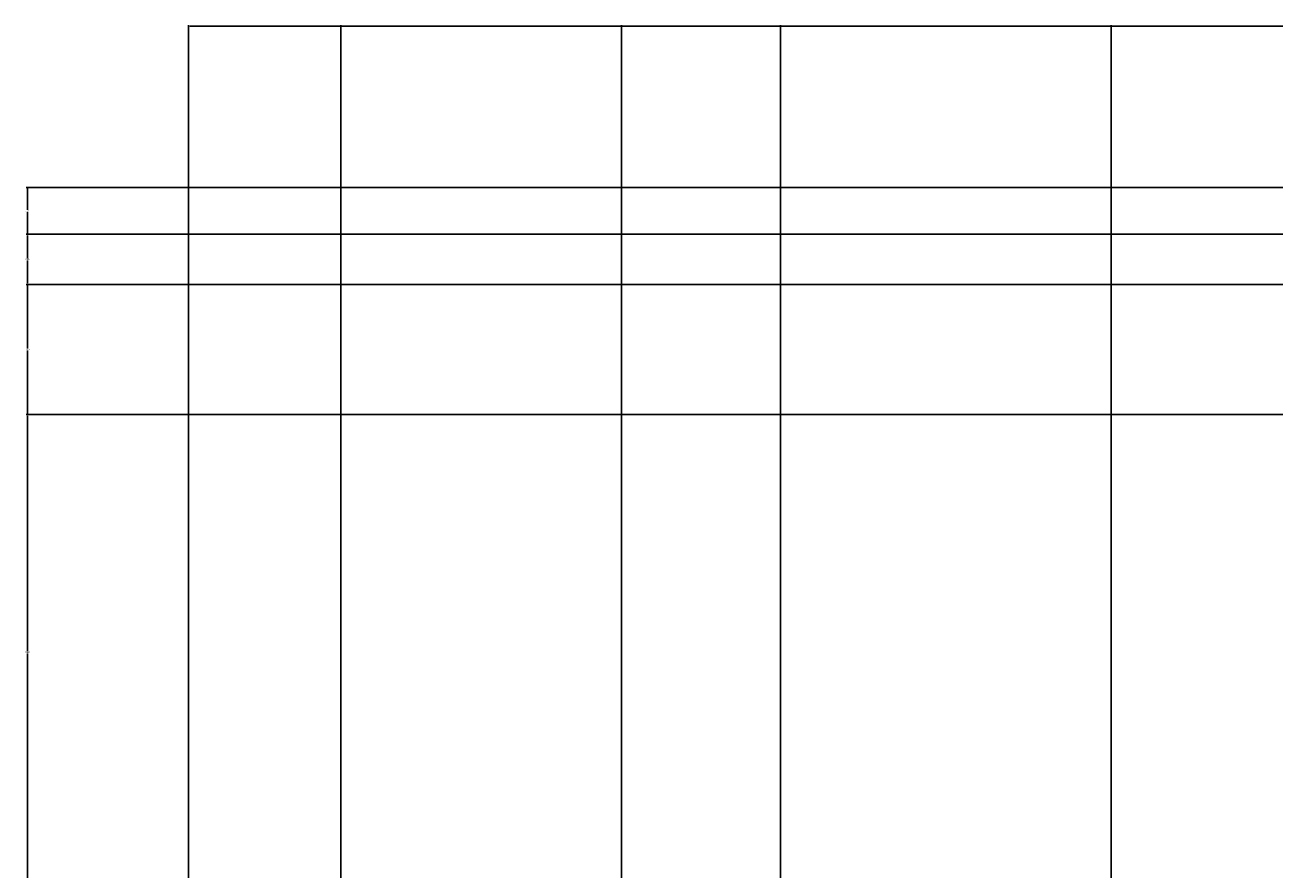
# Model space of a CAD drawing. Units: inches. Extents: x 93 to 565, y 123 to 656.
# Tile 8 of 18: x 93 to 291, y 522 to 656. Entities that reach past the tile are written whole.
import ezdxf

# ---------------------------------------------------------------- set-up
doc = ezdxf.new("R2010")
doc.units = ezdxf.units.IN
doc.header["$MEASUREMENT"] = 0
doc.layers.add('A-ANNO-DIMS', color=2, linetype='Continuous', lineweight=18)
doc.styles.get("Standard").update_dxf_attribs({"font": 'arial.ttf'})
doc.dimstyles.get("Standard").update_dxf_attribs({"dimtxt": 0.18, "dimasz": 0.18, "dimexe": 0.18, "dimexo": 0.0625, "dimgap": 0.09, "dimtad": 0, "dimtih": 1, "dimtoh": 1, "dimdec": 4, "dimzin": 0, "dimdsep": 46, "dimtxsty": 'Standard', "dimcen": 0.09, "dimadec": 0, "dimazin": 0, "dimtfac": 1, "dimtdec": 4, "dimtofl": 0, "dimtmove": 0, "dimatfit": 3, "dimfxl": 1, "dimtolj": 1, "dimtzin": 0, "dimarcsym": 0})

# ---------------------------------------------------------------- blocks, each defined once
blk = doc.blocks.new('*D26')
at = {"layer": 'A-ANNO-DIMS', "color": 0, "lineweight": -2, "transparency": 16777216}
for p, q in [((119.08, 519.16), (119.08, 656.13)), ((119.26, 655.95), (328.79, 655.95)), ((538.9, 655.95), (329.37, 655.95)), ((539.08, 630.47), (539.08, 656.13))]:
    blk.add_line(p, q, dxfattribs=at)
at = {"layer": 'A-ANNO-DIMS', "color": 0, "transparency": 16777216}
for points in [[(119.26, 655.98), (119.26, 655.92), (119.08, 655.95)], [(538.9, 655.98), (538.9, 655.92), (539.08, 655.95)]]:
    blk.add_solid(points, dxfattribs=at)
at = {"layer": 'Defpoints', "color": 0, "transparency": 16777216}
for p in [(539.08, 655.95), (539.08, 630.4), (119.08, 519.1)]:
    blk.add_point(p, dxfattribs=at)
at = {"layer": 'A-ANNO-DIMS', "color": 0, "transparency": 16777216, "insert": (329.08, 655.95), "char_height": 0.18, "attachment_point": 5}
blk.add_mtext('\\A1;420', dxfattribs=at)
blk = doc.blocks.new('*D31')
at = {"layer": 'A-ANNO-DIMS', "color": 0, "lineweight": -2, "transparency": 16777216}
for p, q in [((417.87, 630.4), (564.81, 630.4)), ((564.63, 630.22), (564.63, 395.25)), ((564.63, 159.91), (564.63, 394.89)), ((119.14, 159.73), (564.81, 159.73))]:
    blk.add_line(p, q, dxfattribs=at)
at = {"layer": 'A-ANNO-DIMS', "color": 0, "transparency": 16777216}
for points in [[(564.6, 630.22), (564.66, 630.22), (564.63, 630.4)], [(564.6, 159.91), (564.66, 159.91), (564.63, 159.73)]]:
    blk.add_solid(points, dxfattribs=at)
at = {"layer": 'Defpoints', "color": 0, "transparency": 16777216}
for p in [(417.81, 630.4), (564.63, 630.4), (119.08, 159.73)]:
    blk.add_point(p, dxfattribs=at)
at = {"layer": 'A-ANNO-DIMS', "color": 0, "transparency": 16777216, "insert": (564.63, 395.07), "char_height": 0.18, "attachment_point": 5}
blk.add_mtext('\\A1;470.7', dxfattribs=at)
blk = doc.blocks.new('*D36')
at = {"layer": 'A-ANNO-DIMS', "color": 0, "lineweight": -2, "transparency": 16777216}
for p, q in [((417.75, 594.4), (93.35, 594.4)), ((93.53, 594.22), (93.53, 556.93)), ((93.53, 519.28), (93.53, 556.57)), ((119.02, 519.1), (93.35, 519.1))]:
    blk.add_line(p, q, dxfattribs=at)
at = {"layer": 'A-ANNO-DIMS', "color": 0, "transparency": 16777216}
for points in [[(93.5, 594.22), (93.56, 594.22), (93.53, 594.4)], [(93.5, 519.28), (93.56, 519.28), (93.53, 519.1)]]:
    blk.add_solid(points, dxfattribs=at)
at = {"layer": 'Defpoints', "color": 0, "transparency": 16777216}
for p in [(93.53, 594.4), (417.81, 594.4), (119.08, 519.1)]:
    blk.add_point(p, dxfattribs=at)
at = {"layer": 'A-ANNO-DIMS', "color": 0, "transparency": 16777216, "insert": (93.53, 556.75), "char_height": 0.18, "attachment_point": 5}
blk.add_mtext('\\A1;75.3', dxfattribs=at)
blk = doc.blocks.new('*D49')
at = {"layer": 'A-ANNO-DIMS', "color": 0, "lineweight": -2, "transparency": 16777216}
for p, q in [((119.08, 519.16), (119.08, 656.13)), ((119.26, 655.95), (130.75, 655.95)), ((143.03, 655.95), (131.54, 655.95)), ((143.21, 494.41), (143.21, 656.13))]:
    blk.add_line(p, q, dxfattribs=at)
at = {"layer": 'A-ANNO-DIMS', "color": 0, "transparency": 16777216}
for points in [[(119.26, 655.98), (119.26, 655.92), (119.08, 655.95)], [(143.03, 655.98), (143.03, 655.92), (143.21, 655.95)]]:
    blk.add_solid(points, dxfattribs=at)
at = {"layer": 'Defpoints', "color": 0, "transparency": 16777216}
for p in [(143.21, 655.95), (119.08, 519.1), (143.21, 494.34)]:
    blk.add_point(p, dxfattribs=at)
at = {"layer": 'A-ANNO-DIMS', "color": 0, "transparency": 16777216, "insert": (131.15, 655.95), "char_height": 0.18, "attachment_point": 5}
blk.add_mtext('\\A1;24.13', dxfattribs=at)
blk = doc.blocks.new('*D50')
at = {"layer": 'A-ANNO-DIMS', "color": 0, "lineweight": -2, "transparency": 16777216}
for p, q in [((143.21, 494.41), (143.21, 656.13)), ((143.39, 655.95), (165.03, 655.95)), ((187.47, 655.95), (165.83, 655.95)), ((187.65, 494.41), (187.65, 656.13))]:
    blk.add_line(p, q, dxfattribs=at)
at = {"layer": 'A-ANNO-DIMS', "color": 0, "transparency": 16777216}
for points in [[(143.39, 655.98), (143.39, 655.92), (143.21, 655.95)], [(187.47, 655.98), (187.47, 655.92), (187.65, 655.95)]]:
    blk.add_solid(points, dxfattribs=at)
at = {"layer": 'Defpoints', "color": 0, "transparency": 16777216}
for p in [(187.65, 655.95), (143.21, 494.34), (187.65, 494.34)]:
    blk.add_point(p, dxfattribs=at)
at = {"layer": 'A-ANNO-DIMS', "color": 0, "transparency": 16777216, "insert": (165.43, 655.95), "char_height": 0.18, "attachment_point": 5}
blk.add_mtext('\\A1;44.44', dxfattribs=at)
blk = doc.blocks.new('*D64')
at = {"layer": 'A-ANNO-DIMS', "color": 0, "lineweight": -2, "transparency": 16777216}
for p, q in [((212.83, 427.41), (212.83, 656.13)), ((213.01, 655.95), (238.63, 655.95)), ((265.03, 655.95), (239.41, 655.95)), ((265.21, 427.41), (265.21, 656.13))]:
    blk.add_line(p, q, dxfattribs=at)
at = {"layer": 'A-ANNO-DIMS', "color": 0, "transparency": 16777216}
for points in [[(213.01, 655.98), (213.01, 655.92), (212.83, 655.95)], [(265.03, 655.98), (265.03, 655.92), (265.21, 655.95)]]:
    blk.add_solid(points, dxfattribs=at)
at = {"layer": 'Defpoints', "color": 0, "transparency": 16777216}
for p in [(265.21, 655.95), (212.83, 427.35), (265.21, 427.35)]:
    blk.add_point(p, dxfattribs=at)
at = {"layer": 'A-ANNO-DIMS', "color": 0, "transparency": 16777216, "insert": (239.02, 655.95), "char_height": 0.18, "attachment_point": 5}
blk.add_mtext('\\A1;52.39', dxfattribs=at)
blk = doc.blocks.new('*D94')
at = {"layer": 'A-ANNO-DIMS', "color": 0, "lineweight": -2, "transparency": 16777216}
for p, q in [((423.75, 615.04), (93.35, 615.04)), ((93.53, 614.86), (93.53, 604.9)), ((93.53, 594.58), (93.53, 604.54)), ((417.75, 594.4), (93.35, 594.4))]:
    blk.add_line(p, q, dxfattribs=at)
at = {"layer": 'A-ANNO-DIMS', "color": 0, "transparency": 16777216}
for points in [[(93.5, 614.86), (93.56, 614.86), (93.53, 615.04)], [(93.5, 594.58), (93.56, 594.58), (93.53, 594.4)]]:
    blk.add_solid(points, dxfattribs=at)
at = {"layer": 'Defpoints', "color": 0, "transparency": 16777216}
for p in [(93.53, 615.04), (423.81, 615.04), (417.81, 594.4)]:
    blk.add_point(p, dxfattribs=at)
at = {"layer": 'A-ANNO-DIMS', "color": 0, "transparency": 16777216, "insert": (93.53, 604.72), "char_height": 0.18, "attachment_point": 5}
blk.add_mtext('\\A1;20.636', dxfattribs=at)
blk = doc.blocks.new('*D95')
at = {"layer": 'A-ANNO-DIMS', "color": 0, "lineweight": -2, "transparency": 16777216}
for p, q in [((487.73, 622.97), (93.35, 622.97)), ((93.53, 622.79), (93.53, 619.19)), ((93.53, 615.22), (93.53, 618.82)), ((423.75, 615.04), (93.35, 615.04))]:
    blk.add_line(p, q, dxfattribs=at)
at = {"layer": 'A-ANNO-DIMS', "color": 0, "transparency": 16777216}
for points in [[(93.5, 622.79), (93.56, 622.79), (93.53, 622.97)], [(93.5, 615.22), (93.56, 615.22), (93.53, 615.04)]]:
    blk.add_solid(points, dxfattribs=at)
at = {"layer": 'Defpoints', "color": 0, "transparency": 16777216}
for p in [(93.53, 622.97), (487.8, 622.97), (423.81, 615.04)]:
    blk.add_point(p, dxfattribs=at)
at = {"layer": 'A-ANNO-DIMS', "color": 0, "transparency": 16777216, "insert": (93.53, 619.01), "char_height": 0.18, "attachment_point": 5}
blk.add_mtext('\\A1;7.93', dxfattribs=at)
blk = doc.blocks.new('*D96')
at = {"layer": 'A-ANNO-DIMS', "color": 0, "lineweight": -2, "transparency": 16777216}
for p, q in [((417.75, 630.4), (93.35, 630.4)), ((93.53, 630.22), (93.53, 626.87)), ((93.53, 623.15), (93.53, 626.51)), ((487.73, 622.97), (93.35, 622.97))]:
    blk.add_line(p, q, dxfattribs=at)
at = {"layer": 'A-ANNO-DIMS', "color": 0, "transparency": 16777216}
for points in [[(93.5, 630.22), (93.56, 630.22), (93.53, 630.4)], [(93.5, 623.15), (93.56, 623.15), (93.53, 622.97)]]:
    blk.add_solid(points, dxfattribs=at)
at = {"layer": 'Defpoints', "color": 0, "transparency": 16777216}
for p in [(93.53, 630.4), (417.81, 630.4), (487.8, 622.97)]:
    blk.add_point(p, dxfattribs=at)
at = {"layer": 'A-ANNO-DIMS', "color": 0, "transparency": 16777216, "insert": (93.53, 626.69), "char_height": 0.18, "attachment_point": 5}
blk.add_mtext('\\A1;7.434', dxfattribs=at)
blk = doc.blocks.new('*D105')
at = {"layer": 'A-ANNO-DIMS', "color": 0, "lineweight": -2, "transparency": 16777216}
for p, q in [((119.08, 519.16), (119.08, 656.13)), ((119.26, 655.95), (328.54, 655.95)), ((538.9, 655.95), (329.62, 655.95)), ((539.08, 630.47), (539.08, 656.13))]:
    blk.add_line(p, q, dxfattribs=at)
at = {"layer": 'A-ANNO-DIMS', "color": 0, "transparency": 16777216}
for points in [[(119.26, 655.98), (119.26, 655.92), (119.08, 655.95)], [(538.9, 655.98), (538.9, 655.92), (539.08, 655.95)]]:
    blk.add_solid(points, dxfattribs=at)
at = {"layer": 'Defpoints', "color": 0, "transparency": 16777216}
for p in [(539.08, 655.95), (539.08, 630.4), (119.08, 519.1)]:
    blk.add_point(p, dxfattribs=at)
at = {"layer": 'A-ANNO-DIMS', "color": 0, "transparency": 16777216, "insert": (329.08, 655.95), "char_height": 0.18, "attachment_point": 5}
blk.add_mtext('\\A1;420.000', dxfattribs=at)
blk = doc.blocks.new('*D110')
at = {"layer": 'A-ANNO-DIMS', "color": 0, "lineweight": -2, "transparency": 16777216}
for p, q in [((417.87, 630.4), (564.81, 630.4)), ((564.63, 630.22), (564.63, 395.25)), ((564.63, 159.91), (564.63, 394.89)), ((119.14, 159.73), (564.81, 159.73))]:
    blk.add_line(p, q, dxfattribs=at)
at = {"layer": 'A-ANNO-DIMS', "color": 0, "transparency": 16777216}
for points in [[(564.6, 630.22), (564.66, 630.22), (564.63, 630.4)], [(564.6, 159.91), (564.66, 159.91), (564.63, 159.73)]]:
    blk.add_solid(points, dxfattribs=at)
at = {"layer": 'Defpoints', "color": 0, "transparency": 16777216}
for p in [(417.81, 630.4), (564.63, 630.4), (119.08, 159.73)]:
    blk.add_point(p, dxfattribs=at)
at = {"layer": 'A-ANNO-DIMS', "color": 0, "transparency": 16777216, "insert": (564.63, 395.07), "char_height": 0.18, "attachment_point": 5}
blk.add_mtext('\\A1;470.673', dxfattribs=at)
blk = doc.blocks.new('*D115')
at = {"layer": 'A-ANNO-DIMS', "color": 0, "lineweight": -2, "transparency": 16777216}
for p, q in [((417.75, 594.4), (93.35, 594.4)), ((93.53, 594.22), (93.53, 556.93)), ((93.53, 519.28), (93.53, 556.57)), ((119.02, 519.1), (93.35, 519.1))]:
    blk.add_line(p, q, dxfattribs=at)
at = {"layer": 'A-ANNO-DIMS', "color": 0, "transparency": 16777216}
for points in [[(93.5, 594.22), (93.56, 594.22), (93.53, 594.4)], [(93.5, 519.28), (93.56, 519.28), (93.53, 519.1)]]:
    blk.add_solid(points, dxfattribs=at)
at = {"layer": 'Defpoints', "color": 0, "transparency": 16777216}
for p in [(93.53, 594.4), (417.81, 594.4), (119.08, 519.1)]:
    blk.add_point(p, dxfattribs=at)
at = {"layer": 'A-ANNO-DIMS', "color": 0, "transparency": 16777216, "insert": (93.53, 556.75), "char_height": 0.18, "attachment_point": 5}
blk.add_mtext('\\A1;75.305', dxfattribs=at)
blk = doc.blocks.new('*D128')
at = {"layer": 'A-ANNO-DIMS', "color": 0, "lineweight": -2, "transparency": 16777216}
for p, q in [((119.08, 519.16), (119.08, 656.13)), ((119.26, 655.95), (130.68, 655.95)), ((143.03, 655.95), (131.61, 655.95)), ((143.21, 494.41), (143.21, 656.13))]:
    blk.add_line(p, q, dxfattribs=at)
at = {"layer": 'A-ANNO-DIMS', "color": 0, "transparency": 16777216}
for points in [[(119.26, 655.98), (119.26, 655.92), (119.08, 655.95)], [(143.03, 655.98), (143.03, 655.92), (143.21, 655.95)]]:
    blk.add_solid(points, dxfattribs=at)
at = {"layer": 'Defpoints', "color": 0, "transparency": 16777216}
for p in [(143.21, 655.95), (119.08, 519.1), (143.21, 494.34)]:
    blk.add_point(p, dxfattribs=at)
at = {"layer": 'A-ANNO-DIMS', "color": 0, "transparency": 16777216, "insert": (131.15, 655.95), "char_height": 0.18, "attachment_point": 5}
blk.add_mtext('\\A1;24.132', dxfattribs=at)
blk = doc.blocks.new('*D129')
at = {"layer": 'A-ANNO-DIMS', "color": 0, "lineweight": -2, "transparency": 16777216}
for p, q in [((143.21, 494.41), (143.21, 656.13)), ((143.39, 655.95), (164.96, 655.95)), ((187.47, 655.95), (165.9, 655.95)), ((187.65, 494.41), (187.65, 656.13))]:
    blk.add_line(p, q, dxfattribs=at)
at = {"layer": 'A-ANNO-DIMS', "color": 0, "transparency": 16777216}
for points in [[(143.39, 655.98), (143.39, 655.92), (143.21, 655.95)], [(187.47, 655.98), (187.47, 655.92), (187.65, 655.95)]]:
    blk.add_solid(points, dxfattribs=at)
at = {"layer": 'Defpoints', "color": 0, "transparency": 16777216}
for p in [(187.65, 655.95), (143.21, 494.34), (187.65, 494.34)]:
    blk.add_point(p, dxfattribs=at)
at = {"layer": 'A-ANNO-DIMS', "color": 0, "transparency": 16777216, "insert": (165.43, 655.95), "char_height": 0.18, "attachment_point": 5}
blk.add_mtext('\\A1;44.436', dxfattribs=at)
blk = doc.blocks.new('*D143')
at = {"layer": 'A-ANNO-DIMS', "color": 0, "lineweight": -2, "transparency": 16777216}
for p, q in [((212.83, 427.41), (212.83, 656.13)), ((213.01, 655.95), (238.56, 655.95)), ((265.03, 655.95), (239.48, 655.95)), ((265.21, 427.41), (265.21, 656.13))]:
    blk.add_line(p, q, dxfattribs=at)
at = {"layer": 'A-ANNO-DIMS', "color": 0, "transparency": 16777216}
for points in [[(213.01, 655.98), (213.01, 655.92), (212.83, 655.95)], [(265.03, 655.98), (265.03, 655.92), (265.21, 655.95)]]:
    blk.add_solid(points, dxfattribs=at)
at = {"layer": 'Defpoints', "color": 0, "transparency": 16777216}
for p in [(265.21, 655.95), (212.83, 427.35), (265.21, 427.35)]:
    blk.add_point(p, dxfattribs=at)
at = {"layer": 'A-ANNO-DIMS', "color": 0, "transparency": 16777216, "insert": (239.02, 655.95), "char_height": 0.18, "attachment_point": 5}
blk.add_mtext('\\A1;52.388', dxfattribs=at)
blk = doc.blocks.new('*D173')
at = {"layer": 'A-ANNO-DIMS', "color": 0, "lineweight": -2, "transparency": 16777216}
for p, q in [((423.75, 615.04), (93.35, 615.04)), ((93.53, 614.86), (93.53, 604.9)), ((93.53, 594.58), (93.53, 604.54)), ((417.75, 594.4), (93.35, 594.4))]:
    blk.add_line(p, q, dxfattribs=at)
at = {"layer": 'A-ANNO-DIMS', "color": 0, "transparency": 16777216}
for points in [[(93.5, 614.86), (93.56, 614.86), (93.53, 615.04)], [(93.5, 594.58), (93.56, 594.58), (93.53, 594.4)]]:
    blk.add_solid(points, dxfattribs=at)
at = {"layer": 'Defpoints', "color": 0, "transparency": 16777216}
for p in [(93.53, 615.04), (423.81, 615.04), (417.81, 594.4)]:
    blk.add_point(p, dxfattribs=at)
at = {"layer": 'A-ANNO-DIMS', "color": 0, "transparency": 16777216, "insert": (93.53, 604.72), "char_height": 0.18, "attachment_point": 5}
blk.add_mtext('\\A1;20.636', dxfattribs=at)
blk = doc.blocks.new('*D174')
at = {"layer": 'A-ANNO-DIMS', "color": 0, "lineweight": -2, "transparency": 16777216}
for p, q in [((487.73, 622.97), (93.35, 622.97)), ((93.53, 622.79), (93.53, 619.19)), ((93.53, 615.22), (93.53, 618.82)), ((423.75, 615.04), (93.35, 615.04))]:
    blk.add_line(p, q, dxfattribs=at)
at = {"layer": 'A-ANNO-DIMS', "color": 0, "transparency": 16777216}
for points in [[(93.5, 622.79), (93.56, 622.79), (93.53, 622.97)], [(93.5, 615.22), (93.56, 615.22), (93.53, 615.04)]]:
    blk.add_solid(points, dxfattribs=at)
at = {"layer": 'Defpoints', "color": 0, "transparency": 16777216}
for p in [(93.53, 622.97), (487.8, 622.97), (423.81, 615.04)]:
    blk.add_point(p, dxfattribs=at)
at = {"layer": 'A-ANNO-DIMS', "color": 0, "transparency": 16777216, "insert": (93.53, 619.01), "char_height": 0.18, "attachment_point": 5}
blk.add_mtext('\\A1;7.930', dxfattribs=at)
blk = doc.blocks.new('*D175')
at = {"layer": 'A-ANNO-DIMS', "color": 0, "lineweight": -2, "transparency": 16777216}
for p, q in [((417.75, 630.4), (93.35, 630.4)), ((93.53, 630.22), (93.53, 626.87)), ((93.53, 623.15), (93.53, 626.51)), ((487.73, 622.97), (93.35, 622.97))]:
    blk.add_line(p, q, dxfattribs=at)
at = {"layer": 'A-ANNO-DIMS', "color": 0, "transparency": 16777216}
for points in [[(93.5, 630.22), (93.56, 630.22), (93.53, 630.4)], [(93.5, 623.15), (93.56, 623.15), (93.53, 622.97)]]:
    blk.add_solid(points, dxfattribs=at)
at = {"layer": 'Defpoints', "color": 0, "transparency": 16777216}
for p in [(93.53, 630.4), (417.81, 630.4), (487.8, 622.97)]:
    blk.add_point(p, dxfattribs=at)
at = {"layer": 'A-ANNO-DIMS', "color": 0, "transparency": 16777216, "insert": (93.53, 626.69), "char_height": 0.18, "attachment_point": 5}
blk.add_mtext('\\A1;7.434', dxfattribs=at)

msp = doc.modelspace()

# ---------------------------------------------------------------- dimensions: what is measured, and where the dimension line sits
at = {"layer": 'A-ANNO-DIMS'}
for base, p1, p2, override, picture, middle in [((539.0794, 655.9548), (119.0794, 519.0999), (539.0794, 630.4048), {"dimdec": 0, "dimlfac": 1, "dimrnd": 0, "dimzin": 0, "dimdsep": 46, "dimlunit": 2}, '*D26', (329.0794, 655.9548)), ((143.2118, 655.9548), (119.0794, 519.0999), (143.2118, 494.3434), {"dimdec": 2, "dimlfac": 1, "dimrnd": 0, "dimzin": 0, "dimdsep": 46, "dimlunit": 2}, '*D49', (131.1456, 655.9548)), ((539.0794, 655.9548), (119.0794, 519.0999), (539.0794, 630.4048), {"dimdec": 3, "dimlfac": 1, "dimrnd": 0, "dimzin": 0, "dimdsep": 46, "dimlunit": 2}, '*D105', (329.0794, 655.9548)), ((143.2118, 655.9548), (119.0794, 519.0999), (143.2118, 494.3434), {"dimdec": 3, "dimlfac": 1, "dimrnd": 0, "dimzin": 0, "dimdsep": 46, "dimlunit": 2}, '*D128', (131.1456, 655.9548)), ((187.648, 655.9548), (143.2118, 494.3434), (187.648, 494.3434), {"dimdec": 2, "dimlfac": 1, "dimrnd": 0, "dimzin": 0, "dimdsep": 46, "dimlunit": 2}, '*D50', (165.4299, 655.9548)), ((187.648, 655.9548), (143.2118, 494.3434), (187.648, 494.3434), {"dimdec": 3, "dimlfac": 1, "dimrnd": 0, "dimzin": 0, "dimdsep": 46, "dimlunit": 2}, '*D129', (165.4299, 655.9548)), ((265.2145, 655.9548), (212.8266, 427.3478), (265.2145, 427.3478), {"dimdec": 2, "dimlfac": 1, "dimrnd": 0, "dimzin": 0, "dimdsep": 46, "dimlunit": 2}, '*D64', (239.0206, 655.9548)), ((265.2145, 655.9548), (212.8266, 427.3478), (265.2145, 427.3478), {"dimdec": 3, "dimlfac": 1, "dimrnd": 0, "dimzin": 0, "dimdsep": 46, "dimlunit": 2}, '*D143', (239.0206, 655.9548))]:
    dim = msp.add_linear_dim(base=base, p1=p1, p2=p2, dimstyle='Standard', override=override, dxfattribs=at)
    dim.commit()
    dim.dimension.update_dxf_attribs({"geometry": picture, "text_midpoint": middle})
for base, p1, p2, override, picture, middle in [((93.5294, 630.4048), (487.7953, 622.9711), (417.8097, 630.4048), {"dimdec": 3, "dimlfac": 1, "dimrnd": 0, "dimzin": 0, "dimdsep": 46, "dimlunit": 2}, '*D96', (93.5294, 626.6879)), ((93.5294, 630.4048), (487.7953, 622.9711), (417.8097, 630.4048), {"dimdec": 3, "dimlfac": 1, "dimrnd": 0, "dimzin": 0, "dimdsep": 46, "dimlunit": 2}, '*D175', (93.5294, 626.6879)), ((564.6294, 630.4048), (119.0794, 159.7323), (417.8097, 630.4048), {"dimdec": 1, "dimlfac": 1, "dimrnd": 0, "dimzin": 0, "dimdsep": 46, "dimlunit": 2}, '*D31', (564.6294, 395.0685)), ((564.62936, 630.40478), (119.07936, 159.73225), (417.80971, 630.40477), {"dimdec": 3, "dimlfac": 1, "dimrnd": 0, "dimzin": 0, "dimdsep": 46, "dimlunit": 2}, '*D110', (564.62936, 395.06851)), ((93.52936, 622.97108), (423.80971, 615.0406), (487.79526, 622.97108), {"dimdec": 3, "dimlfac": 1, "dimrnd": 0, "dimzin": 0, "dimdsep": 46, "dimlunit": 2}, '*D174', (93.52936, 619.00584)), ((93.5294, 622.9711), (423.8097, 615.0406), (487.7953, 622.9711), {"dimdec": 2, "dimlfac": 1, "dimrnd": 0, "dimzin": 0, "dimdsep": 46, "dimlunit": 2}, '*D95', (93.5294, 619.0058)), ((93.5294, 615.0406), (417.8097, 594.4048), (423.8097, 615.0406), {"dimdec": 3, "dimlfac": 1, "dimrnd": 0, "dimzin": 0, "dimdsep": 46, "dimlunit": 2}, '*D94', (93.5294, 604.7227)), ((93.5294, 615.0406), (417.8097, 594.4048), (423.8097, 615.0406), {"dimdec": 3, "dimlfac": 1, "dimrnd": 0, "dimzin": 0, "dimdsep": 46, "dimlunit": 2}, '*D173', (93.5294, 604.7227)), ((93.5294, 594.4048), (119.0794, 519.0999), (417.8097, 594.4048), {"dimdec": 3, "dimlfac": 1, "dimrnd": 0, "dimzin": 0, "dimdsep": 46, "dimlunit": 2}, '*D115', (93.5294, 556.7523)), ((93.5294, 594.4048), (119.0794, 519.0999), (417.8097, 594.4048), {"dimdec": 1, "dimlfac": 1, "dimrnd": 0, "dimzin": 0, "dimdsep": 46, "dimlunit": 2}, '*D36', (93.5294, 556.7523))]:
    dim = msp.add_linear_dim(base=base, p1=p1, p2=p2, angle=90, dimstyle='Standard', override=override, dxfattribs=at)
    dim.commit()
    dim.dimension.update_dxf_attribs({"geometry": picture, "text_midpoint": middle})

doc.saveas('drawing.dxf')
